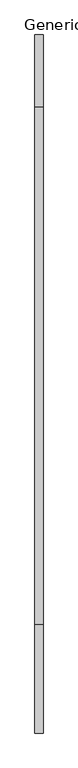
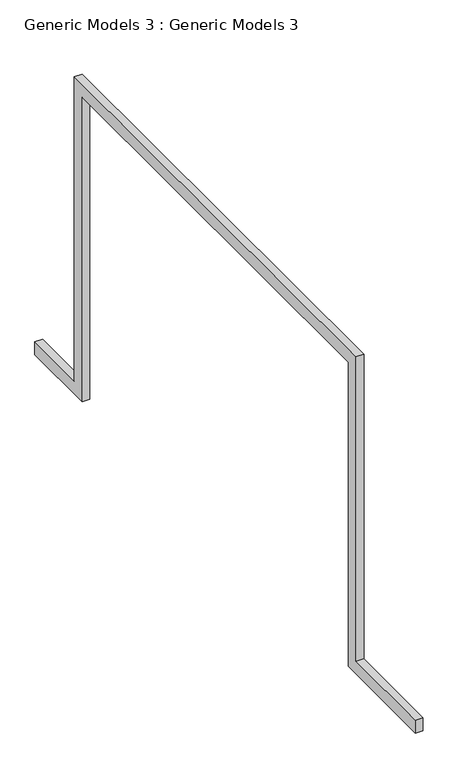
"""IFC4 building model written with IfcOpenShell, lengths in millimetres: proxy geometry, Generic Models 3 : Generic Models 3."""

from ifc_helpers import new_model, si_unit, frame, origin, place, context, project, spatial, polyline, outline, extrude, source, transform, mapped, element, save


def generic_models_3_generic_models_3_794cf474(model_context):
    return source(origin(), model_context, "Body", "SweptSolid", [
        extrude(outline(polyline([(-9452.2396616, 2743.2), (-12878.202305, 2743.2), (-12878.202305, 352.9993493), (-13741.702955, 352.9993493), (-13741.702955, 454.5993493), (-12979.802305, 454.5993493), (-12979.802305, 2844.8), (-9350.6396616, 2844.8), (-9350.6396616, 454.5993493), (-8842.6396616, 454.5993493), (-8842.6396616, 352.9993493), (-9452.2396616, 352.9993493), (-9452.2396616, 2743.2)])), frame((-11853.0273759, 0.0, 0.0), z_axis=(1.0, 0.0, 0.0), x_axis=(0.0, 1.0, 0.0)), (0.0, 0.0, 1.0), 56.7980158),
    ])


if __name__ == "__main__":
    model = new_model("IFC4")
    model_context = context("Model", 3, world=origin())
    ifc_project = project(units=[si_unit("LENGTHUNIT", "METRE", prefix="MILLI")], contexts=[model_context])
    site = spatial("IfcSite", under=ifc_project)
    building = spatial("IfcBuilding", under=site)
    placement = place(None, origin())
    generic_models_3_generic_models_3_shape = generic_models_3_generic_models_3_794cf474(model_context)
    element("IfcBuildingElementProxy", 1, Name="Generic Models 3 : Generic Models 3", ObjectType="Generic Models 3 : Generic Models 3", at=placement, inside=building, context=model_context, shape_type="MappedRepresentation", body=[
        mapped(generic_models_3_generic_models_3_shape, transform((0.0, 0.0, 0.0), x_axis=(1.0, 0.0, 0.0), y_axis=(0.0, 1.0, 0.0), z_axis=(0.0, 0.0, 1.0))),
    ])
    save(model, "model.ifc")

# Revit data of these elements
# Element 1 (IfcBuildingElementProxy, "Generic Models 3 : Generic Models 3")
#   Materials on its faces: "white colour"
# Materials
#   "white colour": class "Generic", colour RGB 120 120 120, transparency 0, Cost = 0
